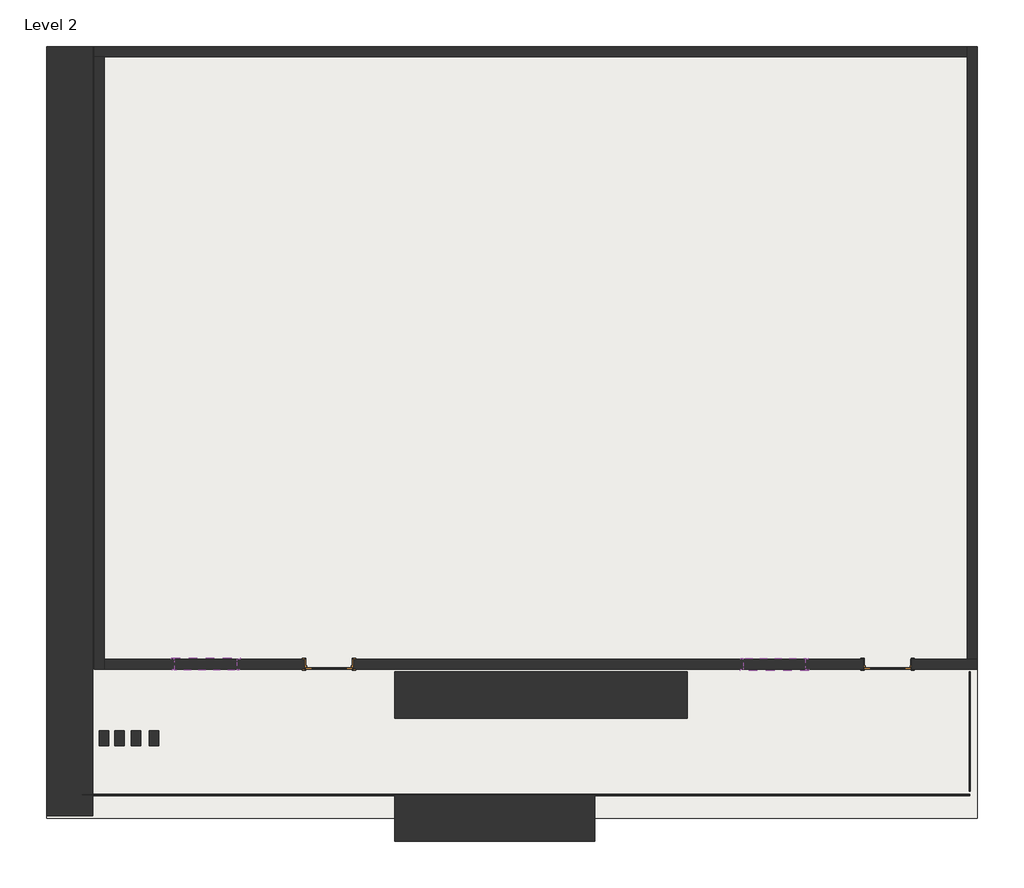
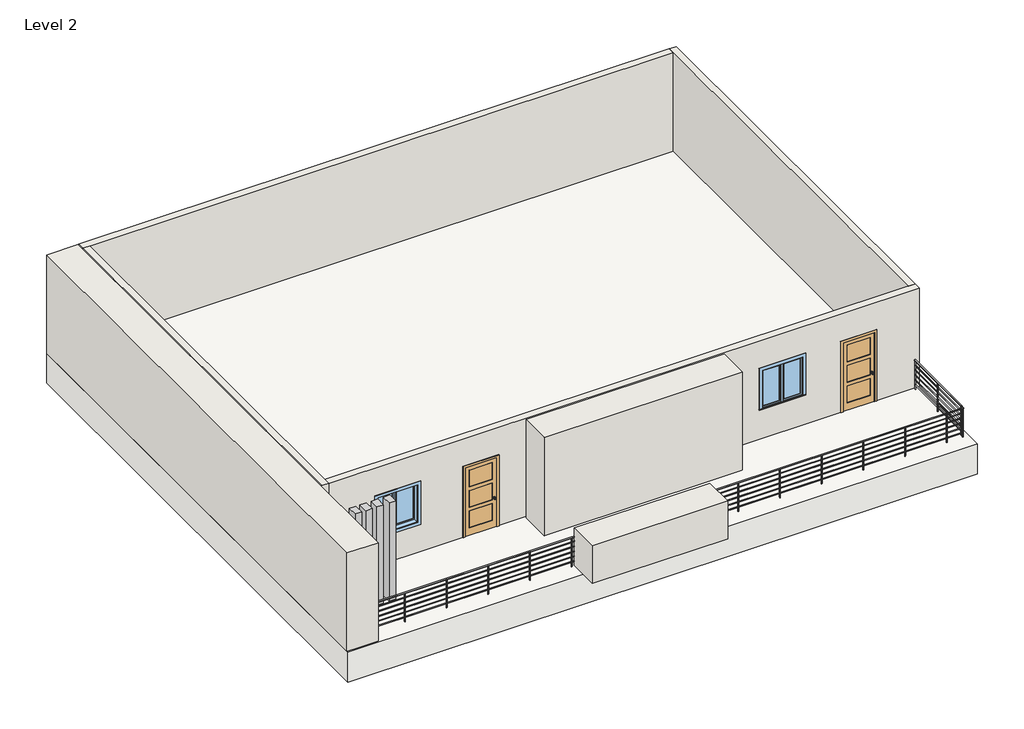
# One storey: 7 walls, 4 columns, 2 doors, 2 railings, 2 windows, 1 slab.
"""IFC4 building model written with IfcOpenShell, lengths in millimetres."""

from ifc_helpers import new_model, si_unit, point, frame, frame_2d, origin, place, context, project, spatial, polyline, circle_curve, trimmed, segment, composite_curve, outline, extrude, faceted_brep, transform, mapped, element, save
from components import wood_timber_column_8_x_12_4a74a8f5, door_54d869bf, window_3a1167bf, window_0862ab64

model = new_model("IFC4")

# Units and contexts
model_context = context("Model", 3, world=origin())
ifc_project = project(units=[si_unit("LENGTHUNIT", "METRE", prefix="MILLI")], contexts=[model_context])

# Site, building, storey
site = spatial("IfcSite", under=ifc_project)
building = spatial("IfcBuilding", under=site)
storey = spatial("IfcBuildingStorey", under=building, Name="Level 2", Elevation=3048.0)

# Columns
placement = place(None, origin())
wood_timber_column_8_x_12_shape = wood_timber_column_8_x_12_4a74a8f5(model_context)
element("IfcColumn", 1, ObjectType="Wood Timber Column : 8 x 12", at=placement, inside=storey, context=model_context, shape_type="MappedRepresentation", body=[
    mapped(wood_timber_column_8_x_12_shape, transform((-18270.7121948, 4590.8323495, 0.0), x_axis=(1.0, 0.0, 0.0), y_axis=(0.0, 1.0, 0.0), z_axis=(0.0, 0.0, 1.0))),
])
element("IfcColumn", 2, ObjectType="Wood Timber Column : 8 x 12", at=placement, inside=storey, context=model_context, shape_type="MappedRepresentation", body=[
    mapped(wood_timber_column_8_x_12_shape, transform((-18600.9121948, 4590.8323495, 0.0), x_axis=(1.0, 0.0, 0.0), y_axis=(0.0, 1.0, 0.0), z_axis=(0.0, 0.0, 1.0))),
])
element("IfcColumn", 3, ObjectType="Wood Timber Column : 8 x 12", at=placement, inside=storey, context=model_context, shape_type="MappedRepresentation", body=[
    mapped(wood_timber_column_8_x_12_shape, transform((-18905.7121948, 4590.8323495, 0.0), x_axis=(1.0, 0.0, 0.0), y_axis=(0.0, 1.0, 0.0), z_axis=(0.0, 0.0, 1.0))),
])
element("IfcColumn", 4, ObjectType="Wood Timber Column : 8 x 12", at=placement, inside=storey, context=model_context, shape_type="MappedRepresentation", body=[
    mapped(wood_timber_column_8_x_12_shape, transform((-17915.1121948, 4590.8323495, 0.0), x_axis=(1.0, 0.0, 0.0), y_axis=(0.0, 1.0, 0.0), z_axis=(0.0, 0.0, 1.0))),
])

# Doors
door_shape = door_54d869bf(model_context)
element("IfcDoor", 5, ObjectType="Door-Interior-Single-3_Panel_Vert-Wood : 36\" x 84\" 2", at=placement, inside=storey, context=model_context, shape_type="MappedRepresentation", body=[
    mapped(door_shape, transform((-3405.3621948, 6054.574368, 3946.3794859), x_axis=(-1.0, 0.0, 0.0), y_axis=(0.0, -1.0, 0.0), z_axis=(0.0, 0.0, 1.0))),
])
element("IfcDoor", 6, ObjectType="Door-Interior-Single-3_Panel_Vert-Wood : 36\" x 84\" 2", at=placement, inside=storey, context=model_context, shape_type="MappedRepresentation", body=[
    mapped(door_shape, transform((-14454.3621948, 6054.574368, 3946.3794859), x_axis=(-1.0, 0.0, 0.0), y_axis=(0.0, -1.0, 0.0), z_axis=(0.0, 0.0, 1.0))),
])

# Railings
element("IfcRailing", 7, ObjectType="Handrail - Pipe", at=placement, inside=storey, context=model_context, shape_type="SweptSolid", body=[
    extrude(outline(composite_curve([segment(trimmed(circle_curve(frame_2d((3466.949368, 4841.7294859)), 19.05), [point((3447.899368, 4841.7294859))], [point((3485.999368, 4841.7294859))], False, "CARTESIAN"), True, "CONTINUOUS"), segment(trimmed(circle_curve(frame_2d((3466.949368, 4841.7294859)), 19.05), [point((3485.999368, 4841.7294859))], [point((3447.899368, 4841.7294859))], False, "CARTESIAN"), True, "CONTINUOUS")], self_intersect=False)), frame((-19331.1621948, 0.0, 0.0), z_axis=(1.0, 0.0, 0.0), x_axis=(0.0, 1.0, 0.0)), (0.0, 0.0, 1.0), 17551.4),
    extrude(outline(composite_curve([segment(trimmed(circle_curve(frame_2d((3466.949368, 4695.6794859)), 12.7), [point((3479.649368, 4695.6794859))], [point((3454.249368, 4695.6794859))], False, "CARTESIAN"), True, "CONTINUOUS"), segment(trimmed(circle_curve(frame_2d((3466.949368, 4695.6794859)), 12.7), [point((3454.249368, 4695.6794859))], [point((3479.649368, 4695.6794859))], False, "CARTESIAN"), True, "CONTINUOUS")], self_intersect=False)), frame((-19331.1621948, 0.0, 0.0), z_axis=(1.0, 0.0, 0.0), x_axis=(0.0, 1.0, 0.0)), (0.0, 0.0, 1.0), 17551.4),
    extrude(outline(composite_curve([segment(trimmed(circle_curve(frame_2d((3466.949368, 4543.2794859)), 12.7), [point((3479.649368, 4543.2794859))], [point((3454.249368, 4543.2794859))], False, "CARTESIAN"), True, "CONTINUOUS"), segment(trimmed(circle_curve(frame_2d((3466.949368, 4543.2794859)), 12.7), [point((3454.249368, 4543.2794859))], [point((3479.649368, 4543.2794859))], False, "CARTESIAN"), True, "CONTINUOUS")], self_intersect=False)), frame((-19331.1621948, 0.0, 0.0), z_axis=(1.0, 0.0, 0.0), x_axis=(0.0, 1.0, 0.0)), (0.0, 0.0, 1.0), 17551.4),
    extrude(outline(composite_curve([segment(trimmed(circle_curve(frame_2d((3466.949368, 4390.8794859)), 12.7), [point((3479.649368, 4390.8794859))], [point((3454.249368, 4390.8794859))], False, "CARTESIAN"), True, "CONTINUOUS"), segment(trimmed(circle_curve(frame_2d((3466.949368, 4390.8794859)), 12.7), [point((3454.249368, 4390.8794859))], [point((3479.649368, 4390.8794859))], False, "CARTESIAN"), True, "CONTINUOUS")], self_intersect=False)), frame((-19331.1621948, 0.0, 0.0), z_axis=(1.0, 0.0, 0.0), x_axis=(0.0, 1.0, 0.0)), (0.0, 0.0, 1.0), 17551.4),
    extrude(outline(composite_curve([segment(trimmed(circle_curve(frame_2d((3466.949368, 4238.4794859)), 12.7), [point((3479.649368, 4238.4794859))], [point((3454.249368, 4238.4794859))], False, "CARTESIAN"), True, "CONTINUOUS"), segment(trimmed(circle_curve(frame_2d((3466.949368, 4238.4794859)), 12.7), [point((3454.249368, 4238.4794859))], [point((3479.649368, 4238.4794859))], False, "CARTESIAN"), True, "CONTINUOUS")], self_intersect=False)), frame((-19331.1621948, 0.0, 0.0), z_axis=(1.0, 0.0, 0.0), x_axis=(0.0, 1.0, 0.0)), (0.0, 0.0, 1.0), 17551.4),
    extrude(outline(composite_curve([segment(trimmed(circle_curve(frame_2d((3466.949368, 4086.0794859)), 12.7), [point((3479.649368, 4086.0794859))], [point((3454.249368, 4086.0794859))], False, "CARTESIAN"), True, "CONTINUOUS"), segment(trimmed(circle_curve(frame_2d((3466.949368, 4086.0794859)), 12.7), [point((3454.249368, 4086.0794859))], [point((3479.649368, 4086.0794859))], False, "CARTESIAN"), True, "CONTINUOUS")], self_intersect=False)), frame((-19331.1621948, 0.0, 0.0), z_axis=(1.0, 0.0, 0.0), x_axis=(0.0, 1.0, 0.0)), (0.0, 0.0, 1.0), 17551.4),
    extrude(outline(composite_curve([segment(trimmed(circle_curve(frame_2d((-2262.3621948, 3466.949368)), 12.7), [point((-2262.3621948, 3479.649368))], [point((-2262.3621948, 3454.249368))], False, "CARTESIAN"), True, "CONTINUOUS"), segment(trimmed(circle_curve(frame_2d((-2262.3621948, 3466.949368)), 12.7), [point((-2262.3621948, 3454.249368))], [point((-2262.3621948, 3479.649368))], False, "CARTESIAN"), True, "CONTINUOUS")], self_intersect=False)), frame((0.0, 0.0, 3946.3794859), z_axis=(0.0, 0.0, 1.0), x_axis=(1.0, 0.0, 0.0)), (0.0, 0.0, 1.0), 876.3),
    extrude(outline(composite_curve([segment(trimmed(circle_curve(frame_2d((-3481.5621948, 3466.949368)), 12.7), [point((-3481.5621948, 3479.649368))], [point((-3481.5621948, 3454.249368))], False, "CARTESIAN"), True, "CONTINUOUS"), segment(trimmed(circle_curve(frame_2d((-3481.5621948, 3466.949368)), 12.7), [point((-3481.5621948, 3454.249368))], [point((-3481.5621948, 3479.649368))], False, "CARTESIAN"), True, "CONTINUOUS")], self_intersect=False)), frame((0.0, 0.0, 3946.3794859), z_axis=(0.0, 0.0, 1.0), x_axis=(1.0, 0.0, 0.0)), (0.0, 0.0, 1.0), 876.3),
    extrude(outline(composite_curve([segment(trimmed(circle_curve(frame_2d((-4700.7621948, 3466.949368)), 12.7), [point((-4700.7621948, 3479.649368))], [point((-4700.7621948, 3454.249368))], False, "CARTESIAN"), True, "CONTINUOUS"), segment(trimmed(circle_curve(frame_2d((-4700.7621948, 3466.949368)), 12.7), [point((-4700.7621948, 3454.249368))], [point((-4700.7621948, 3479.649368))], False, "CARTESIAN"), True, "CONTINUOUS")], self_intersect=False)), frame((0.0, 0.0, 3946.3794859), z_axis=(0.0, 0.0, 1.0), x_axis=(1.0, 0.0, 0.0)), (0.0, 0.0, 1.0), 876.3),
    extrude(outline(composite_curve([segment(trimmed(circle_curve(frame_2d((-5919.9621948, 3466.949368)), 12.7), [point((-5919.9621948, 3479.649368))], [point((-5919.9621948, 3454.249368))], False, "CARTESIAN"), True, "CONTINUOUS"), segment(trimmed(circle_curve(frame_2d((-5919.9621948, 3466.949368)), 12.7), [point((-5919.9621948, 3454.249368))], [point((-5919.9621948, 3479.649368))], False, "CARTESIAN"), True, "CONTINUOUS")], self_intersect=False)), frame((0.0, 0.0, 3946.3794859), z_axis=(0.0, 0.0, 1.0), x_axis=(1.0, 0.0, 0.0)), (0.0, 0.0, 1.0), 876.3),
    extrude(outline(composite_curve([segment(trimmed(circle_curve(frame_2d((-7139.1621948, 3466.949368)), 12.7), [point((-7139.1621948, 3479.649368))], [point((-7139.1621948, 3454.249368))], False, "CARTESIAN"), True, "CONTINUOUS"), segment(trimmed(circle_curve(frame_2d((-7139.1621948, 3466.949368)), 12.7), [point((-7139.1621948, 3454.249368))], [point((-7139.1621948, 3479.649368))], False, "CARTESIAN"), True, "CONTINUOUS")], self_intersect=False)), frame((0.0, 0.0, 3946.3794859), z_axis=(0.0, 0.0, 1.0), x_axis=(1.0, 0.0, 0.0)), (0.0, 0.0, 1.0), 876.3),
    extrude(outline(composite_curve([segment(trimmed(circle_curve(frame_2d((-8358.3621948, 3466.949368)), 12.7), [point((-8358.3621948, 3479.649368))], [point((-8358.3621948, 3454.249368))], False, "CARTESIAN"), True, "CONTINUOUS"), segment(trimmed(circle_curve(frame_2d((-8358.3621948, 3466.949368)), 12.7), [point((-8358.3621948, 3454.249368))], [point((-8358.3621948, 3479.649368))], False, "CARTESIAN"), True, "CONTINUOUS")], self_intersect=False)), frame((0.0, 0.0, 3946.3794859), z_axis=(0.0, 0.0, 1.0), x_axis=(1.0, 0.0, 0.0)), (0.0, 0.0, 1.0), 876.3),
    extrude(outline(composite_curve([segment(trimmed(circle_curve(frame_2d((-9577.5621948, 3466.949368)), 12.7), [point((-9577.5621948, 3479.649368))], [point((-9577.5621948, 3454.249368))], False, "CARTESIAN"), True, "CONTINUOUS"), segment(trimmed(circle_curve(frame_2d((-9577.5621948, 3466.949368)), 12.7), [point((-9577.5621948, 3454.249368))], [point((-9577.5621948, 3479.649368))], False, "CARTESIAN"), True, "CONTINUOUS")], self_intersect=False)), frame((0.0, 0.0, 3946.3794859), z_axis=(0.0, 0.0, 1.0), x_axis=(1.0, 0.0, 0.0)), (0.0, 0.0, 1.0), 876.3),
    extrude(outline(composite_curve([segment(trimmed(circle_curve(frame_2d((-10796.7621948, 3466.949368)), 12.7), [point((-10796.7621948, 3479.649368))], [point((-10796.7621948, 3454.249368))], False, "CARTESIAN"), True, "CONTINUOUS"), segment(trimmed(circle_curve(frame_2d((-10796.7621948, 3466.949368)), 12.7), [point((-10796.7621948, 3454.249368))], [point((-10796.7621948, 3479.649368))], False, "CARTESIAN"), True, "CONTINUOUS")], self_intersect=False)), frame((0.0, 0.0, 3946.3794859), z_axis=(0.0, 0.0, 1.0), x_axis=(1.0, 0.0, 0.0)), (0.0, 0.0, 1.0), 876.3),
    extrude(outline(composite_curve([segment(trimmed(circle_curve(frame_2d((-12015.9621948, 3466.949368)), 12.7), [point((-12015.9621948, 3479.649368))], [point((-12015.9621948, 3454.249368))], False, "CARTESIAN"), True, "CONTINUOUS"), segment(trimmed(circle_curve(frame_2d((-12015.9621948, 3466.949368)), 12.7), [point((-12015.9621948, 3454.249368))], [point((-12015.9621948, 3479.649368))], False, "CARTESIAN"), True, "CONTINUOUS")], self_intersect=False)), frame((0.0, 0.0, 3946.3794859), z_axis=(0.0, 0.0, 1.0), x_axis=(1.0, 0.0, 0.0)), (0.0, 0.0, 1.0), 876.3),
    extrude(outline(composite_curve([segment(trimmed(circle_curve(frame_2d((-13235.1621948, 3466.949368)), 12.7), [point((-13235.1621948, 3479.649368))], [point((-13235.1621948, 3454.249368))], False, "CARTESIAN"), True, "CONTINUOUS"), segment(trimmed(circle_curve(frame_2d((-13235.1621948, 3466.949368)), 12.7), [point((-13235.1621948, 3454.249368))], [point((-13235.1621948, 3479.649368))], False, "CARTESIAN"), True, "CONTINUOUS")], self_intersect=False)), frame((0.0, 0.0, 3946.3794859), z_axis=(0.0, 0.0, 1.0), x_axis=(1.0, 0.0, 0.0)), (0.0, 0.0, 1.0), 876.3),
    extrude(outline(composite_curve([segment(trimmed(circle_curve(frame_2d((-14454.3621948, 3466.949368)), 12.7), [point((-14454.3621948, 3479.649368))], [point((-14454.3621948, 3454.249368))], False, "CARTESIAN"), True, "CONTINUOUS"), segment(trimmed(circle_curve(frame_2d((-14454.3621948, 3466.949368)), 12.7), [point((-14454.3621948, 3454.249368))], [point((-14454.3621948, 3479.649368))], False, "CARTESIAN"), True, "CONTINUOUS")], self_intersect=False)), frame((0.0, 0.0, 3946.3794859), z_axis=(0.0, 0.0, 1.0), x_axis=(1.0, 0.0, 0.0)), (0.0, 0.0, 1.0), 876.3),
    extrude(outline(composite_curve([segment(trimmed(circle_curve(frame_2d((-15673.5621948, 3466.949368)), 12.7), [point((-15673.5621948, 3479.649368))], [point((-15673.5621948, 3454.249368))], False, "CARTESIAN"), True, "CONTINUOUS"), segment(trimmed(circle_curve(frame_2d((-15673.5621948, 3466.949368)), 12.7), [point((-15673.5621948, 3454.249368))], [point((-15673.5621948, 3479.649368))], False, "CARTESIAN"), True, "CONTINUOUS")], self_intersect=False)), frame((0.0, 0.0, 3946.3794859), z_axis=(0.0, 0.0, 1.0), x_axis=(1.0, 0.0, 0.0)), (0.0, 0.0, 1.0), 876.3),
    extrude(outline(composite_curve([segment(trimmed(circle_curve(frame_2d((-16892.7621948, 3466.949368)), 12.7), [point((-16892.7621948, 3479.649368))], [point((-16892.7621948, 3454.249368))], False, "CARTESIAN"), True, "CONTINUOUS"), segment(trimmed(circle_curve(frame_2d((-16892.7621948, 3466.949368)), 12.7), [point((-16892.7621948, 3454.249368))], [point((-16892.7621948, 3479.649368))], False, "CARTESIAN"), True, "CONTINUOUS")], self_intersect=False)), frame((0.0, 0.0, 3946.3794859), z_axis=(0.0, 0.0, 1.0), x_axis=(1.0, 0.0, 0.0)), (0.0, 0.0, 1.0), 876.3),
    extrude(outline(composite_curve([segment(trimmed(circle_curve(frame_2d((-18111.9621948, 3466.949368)), 12.7), [point((-18111.9621948, 3479.649368))], [point((-18111.9621948, 3454.249368))], False, "CARTESIAN"), True, "CONTINUOUS"), segment(trimmed(circle_curve(frame_2d((-18111.9621948, 3466.949368)), 12.7), [point((-18111.9621948, 3454.249368))], [point((-18111.9621948, 3479.649368))], False, "CARTESIAN"), True, "CONTINUOUS")], self_intersect=False)), frame((0.0, 0.0, 3946.3794859), z_axis=(0.0, 0.0, 1.0), x_axis=(1.0, 0.0, 0.0)), (0.0, 0.0, 1.0), 876.3),
    extrude(outline(composite_curve([segment(trimmed(circle_curve(frame_2d((-1792.4621948, 3466.949368)), 12.7), [point((-1792.4621948, 3479.649368))], [point((-1792.4621948, 3454.249368))], False, "CARTESIAN"), True, "CONTINUOUS"), segment(trimmed(circle_curve(frame_2d((-1792.4621948, 3466.949368)), 12.7), [point((-1792.4621948, 3454.249368))], [point((-1792.4621948, 3479.649368))], False, "CARTESIAN"), True, "CONTINUOUS")], self_intersect=False)), frame((0.0, 0.0, 3946.3794859), z_axis=(0.0, 0.0, 1.0), x_axis=(1.0, 0.0, 0.0)), (0.0, 0.0, 1.0), 876.3),
    extrude(outline(composite_curve([segment(trimmed(circle_curve(frame_2d((-19318.4621948, 3466.949368)), 12.7), [point((-19318.4621948, 3479.649368))], [point((-19318.4621948, 3454.249368))], False, "CARTESIAN"), True, "CONTINUOUS"), segment(trimmed(circle_curve(frame_2d((-19318.4621948, 3466.949368)), 12.7), [point((-19318.4621948, 3454.249368))], [point((-19318.4621948, 3479.649368))], False, "CARTESIAN"), True, "CONTINUOUS")], self_intersect=False)), frame((0.0, 0.0, 3946.3794859), z_axis=(0.0, 0.0, 1.0), x_axis=(1.0, 0.0, 0.0)), (0.0, 0.0, 1.0), 876.3),
])
element("IfcRailing", 8, ObjectType="Handrail - Pipe", at=placement, inside=storey, context=model_context, shape_type="SweptSolid", body=[
    extrude(outline(composite_curve([segment(trimmed(circle_curve(frame_2d((4841.7294859, -1779.7621948)), 19.05), [point((4841.7294859, -1760.7121948))], [point((4841.7294859, -1798.8121948))], False, "CARTESIAN"), True, "CONTINUOUS"), segment(trimmed(circle_curve(frame_2d((4841.7294859, -1779.7621948)), 19.05), [point((4841.7294859, -1798.8121948))], [point((4841.7294859, -1760.7121948))], False, "CARTESIAN"), True, "CONTINUOUS")], self_intersect=False)), frame((0.0, 3543.149368, 0.0), z_axis=(0.0, 1.0, 0.0), x_axis=(0.0, 0.0, 1.0)), (0.0, 0.0, 1.0), 2362.2),
    extrude(outline(composite_curve([segment(trimmed(circle_curve(frame_2d((4695.6794859, -1779.7621948)), 12.7), [point((4695.6794859, -1792.4621948))], [point((4695.6794859, -1767.0621948))], False, "CARTESIAN"), True, "CONTINUOUS"), segment(trimmed(circle_curve(frame_2d((4695.6794859, -1779.7621948)), 12.7), [point((4695.6794859, -1767.0621948))], [point((4695.6794859, -1792.4621948))], False, "CARTESIAN"), True, "CONTINUOUS")], self_intersect=False)), frame((0.0, 3543.149368, 0.0), z_axis=(0.0, 1.0, 0.0), x_axis=(0.0, 0.0, 1.0)), (0.0, 0.0, 1.0), 2362.2),
    extrude(outline(composite_curve([segment(trimmed(circle_curve(frame_2d((4543.2794859, -1779.7621948)), 12.7), [point((4543.2794859, -1792.4621948))], [point((4543.2794859, -1767.0621948))], False, "CARTESIAN"), True, "CONTINUOUS"), segment(trimmed(circle_curve(frame_2d((4543.2794859, -1779.7621948)), 12.7), [point((4543.2794859, -1767.0621948))], [point((4543.2794859, -1792.4621948))], False, "CARTESIAN"), True, "CONTINUOUS")], self_intersect=False)), frame((0.0, 3543.149368, 0.0), z_axis=(0.0, 1.0, 0.0), x_axis=(0.0, 0.0, 1.0)), (0.0, 0.0, 1.0), 2362.2),
    extrude(outline(composite_curve([segment(trimmed(circle_curve(frame_2d((4390.8794859, -1779.7621948)), 12.7), [point((4390.8794859, -1792.4621948))], [point((4390.8794859, -1767.0621948))], False, "CARTESIAN"), True, "CONTINUOUS"), segment(trimmed(circle_curve(frame_2d((4390.8794859, -1779.7621948)), 12.7), [point((4390.8794859, -1767.0621948))], [point((4390.8794859, -1792.4621948))], False, "CARTESIAN"), True, "CONTINUOUS")], self_intersect=False)), frame((0.0, 3543.149368, 0.0), z_axis=(0.0, 1.0, 0.0), x_axis=(0.0, 0.0, 1.0)), (0.0, 0.0, 1.0), 2362.2),
    extrude(outline(composite_curve([segment(trimmed(circle_curve(frame_2d((4238.4794859, -1779.7621948)), 12.7), [point((4238.4794859, -1792.4621948))], [point((4238.4794859, -1767.0621948))], False, "CARTESIAN"), True, "CONTINUOUS"), segment(trimmed(circle_curve(frame_2d((4238.4794859, -1779.7621948)), 12.7), [point((4238.4794859, -1767.0621948))], [point((4238.4794859, -1792.4621948))], False, "CARTESIAN"), True, "CONTINUOUS")], self_intersect=False)), frame((0.0, 3543.149368, 0.0), z_axis=(0.0, 1.0, 0.0), x_axis=(0.0, 0.0, 1.0)), (0.0, 0.0, 1.0), 2362.2),
    extrude(outline(composite_curve([segment(trimmed(circle_curve(frame_2d((4086.0794859, -1779.7621948)), 12.7), [point((4086.0794859, -1792.4621948))], [point((4086.0794859, -1767.0621948))], False, "CARTESIAN"), True, "CONTINUOUS"), segment(trimmed(circle_curve(frame_2d((4086.0794859, -1779.7621948)), 12.7), [point((4086.0794859, -1767.0621948))], [point((4086.0794859, -1792.4621948))], False, "CARTESIAN"), True, "CONTINUOUS")], self_intersect=False)), frame((0.0, 3543.149368, 0.0), z_axis=(0.0, 1.0, 0.0), x_axis=(0.0, 0.0, 1.0)), (0.0, 0.0, 1.0), 2362.2),
    extrude(outline(composite_curve([segment(trimmed(circle_curve(frame_2d((-1779.7621948, 4762.349368)), 12.7), [point((-1792.4621948, 4762.349368))], [point((-1767.0621948, 4762.349368))], False, "CARTESIAN"), True, "CONTINUOUS"), segment(trimmed(circle_curve(frame_2d((-1779.7621948, 4762.349368)), 12.7), [point((-1767.0621948, 4762.349368))], [point((-1792.4621948, 4762.349368))], False, "CARTESIAN"), True, "CONTINUOUS")], self_intersect=False)), frame((0.0, 0.0, 3946.3794859), z_axis=(0.0, 0.0, 1.0), x_axis=(1.0, 0.0, 0.0)), (0.0, 0.0, 1.0), 876.3),
    extrude(outline(composite_curve([segment(trimmed(circle_curve(frame_2d((-1779.7621948, 5892.649368)), 12.7), [point((-1792.4621948, 5892.649368))], [point((-1767.0621948, 5892.649368))], False, "CARTESIAN"), True, "CONTINUOUS"), segment(trimmed(circle_curve(frame_2d((-1779.7621948, 5892.649368)), 12.7), [point((-1767.0621948, 5892.649368))], [point((-1792.4621948, 5892.649368))], False, "CARTESIAN"), True, "CONTINUOUS")], self_intersect=False)), frame((0.0, 0.0, 3946.3794859), z_axis=(0.0, 0.0, 1.0), x_axis=(1.0, 0.0, 0.0)), (0.0, 0.0, 1.0), 876.3),
    extrude(outline(composite_curve([segment(trimmed(circle_curve(frame_2d((-1779.7621948, 3555.849368)), 12.7), [point((-1792.4621948, 3555.849368))], [point((-1767.0621948, 3555.849368))], False, "CARTESIAN"), True, "CONTINUOUS"), segment(trimmed(circle_curve(frame_2d((-1779.7621948, 3555.849368)), 12.7), [point((-1767.0621948, 3555.849368))], [point((-1792.4621948, 3555.849368))], False, "CARTESIAN"), True, "CONTINUOUS")], self_intersect=False)), frame((0.0, 0.0, 3946.3794859), z_axis=(0.0, 0.0, 1.0), x_axis=(1.0, 0.0, 0.0)), (0.0, 0.0, 1.0), 876.3),
])

# Slab
element("IfcSlab", 9, ObjectType="Generic - 3'", at=placement, inside=storey, context=model_context, shape_type="SweptSolid", body=[
    extrude(outline(polyline([(-1627.3621948, 18275.149368), (-1627.3621948, 3009.749368), (-20042.3621948, 3009.749368), (-20042.3621948, 18275.149368), (-1627.3621948, 18275.149368)])), frame((0.0, 0.0, 3031.9794859), z_axis=(0.0, 0.0, 1.0), x_axis=(1.0, 0.0, 0.0)), (0.0, 0.0, 1.0), 914.4),
])

# Walls
element("IfcWall", 10, ObjectType="Generic - 3' 2", at=placement, inside=storey, context=model_context, shape_type="SweptSolid", body=[
    extrude(outline(polyline([(-7367.7621948, 4990.949368), (-13158.9621948, 4990.949368), (-13158.9621948, 5905.349368), (-7367.7621948, 5905.349368), (-7367.7621948, 4990.949368)])), frame((0.0, 0.0, 3946.3794859), z_axis=(0.0, 0.0, 1.0), x_axis=(1.0, 0.0, 0.0)), (0.0, 0.0, 1.0), 3048.0),
])
element("IfcWall", 11, ObjectType="Generic - 3' 4", at=placement, inside=storey, context=model_context, shape_type="SweptSolid", body=[
    extrude(outline(polyline([(-9196.5621948, 2552.549368), (-13158.9621948, 2552.549368), (-13158.9621948, 3466.949368), (-9196.5621948, 3466.949368), (-9196.5621948, 2552.549368)])), frame((0.0, 0.0, 3946.3794859), z_axis=(0.0, 0.0, 1.0), x_axis=(1.0, 0.0, 0.0)), (0.0, 0.0, 1.0), 1165.3811612),
])
element("IfcWall", 12, ObjectType="Generic - 3' 4", at=placement, inside=storey, context=model_context, shape_type="SweptSolid", body=[
    extrude(outline(polyline([(-20042.3621948, 3060.549368), (-20042.3621948, 18275.149368), (-19127.9621948, 18275.149368), (-19127.9621948, 3060.549368), (-20042.3621948, 3060.549368)])), frame((0.0, 0.0, 3946.3794859), z_axis=(0.0, 0.0, 1.0), x_axis=(1.0, 0.0, 0.0)), (0.0, 0.0, 1.0), 3048.0),
])
element("IfcWall", 13, ObjectType="Generic - 8\"", at=placement, inside=storey, context=model_context, shape_type="Brep", body=[
    faceted_brep([(-19102.5621948, 18071.949368, 3946.3794859), (-18899.3621948, 18071.949368, 3946.3794859), (-1830.5621948, 18071.949368, 3946.3794859), (-1830.5621948, 18071.949368, 6994.3794859), (-18899.3621948, 18071.949368, 6994.3794859), (-19102.5621948, 18071.949368, 6994.3794859), (-19102.5621948, 18275.149368, 3946.3794859), (-19102.5621948, 18275.149368, 6994.3794859), (-1830.5621948, 18275.149368, 6994.3794859), (-1830.5621948, 18275.149368, 3946.3794859)], [[[0, 1, 2, 3, 4, 5]], [[6, 7, 8, 9]], [[2, 1, 0, 6, 9]], [[5, 4, 3, 8, 7]], [[0, 5, 7, 6]], [[3, 2, 9, 8]]]),
])
element("IfcWall", 14, ObjectType="Generic - 8\"", at=placement, inside=storey, context=model_context, shape_type="Brep", body=[
    faceted_brep([(-18899.3621948, 6159.349368, 6994.3794859), (-1830.5621948, 6159.349368, 6994.3794859), (-1627.3621948, 6159.349368, 6994.3794859), (-1627.3621948, 6159.349368, 3946.3794859), (-1830.5621948, 6159.349368, 3946.3794859), (-2922.7621948, 6159.349368, 3946.3794859), (-2922.7621948, 6159.349368, 6105.3794859), (-3887.9621948, 6159.349368, 6105.3794859), (-3887.9621948, 6159.349368, 3946.3794859), (-13971.7621948, 6159.349368, 3946.3794859), (-13971.7621948, 6159.349368, 6105.3794859), (-14936.9621948, 6159.349368, 6105.3794859), (-14936.9621948, 6159.349368, 3946.3794859), (-18899.3621948, 6159.349368, 3946.3794859), (-17502.3621948, 6159.349368, 6079.9794859), (-17502.3621948, 6159.349368, 4860.7794859), (-16283.1621948, 6159.349368, 4860.7794859), (-16283.1621948, 6159.349368, 6079.9794859), (-6250.1621948, 6159.349368, 6079.9794859), (-6250.1621948, 6159.349368, 4860.7794859), (-5030.9621948, 6159.349368, 4860.7794859), (-5030.9621948, 6159.349368, 6079.9794859), (-1627.3621948, 5956.149368, 6994.3794859), (-18899.3621948, 5956.149368, 6994.3794859), (-18899.3621948, 5956.149368, 3946.3794859), (-14936.9621948, 5956.149368, 3946.3794859), (-14936.9621948, 5956.149368, 6105.3794859), (-13971.7621948, 5956.149368, 6105.3794859), (-13971.7621948, 5956.149368, 3946.3794859), (-3887.9621948, 5956.149368, 3946.3794859), (-3887.9621948, 5956.149368, 6105.3794859), (-2922.7621948, 5956.149368, 6105.3794859), (-2922.7621948, 5956.149368, 3946.3794859), (-1627.3621948, 5956.149368, 3946.3794859), (-17502.3621948, 5956.149368, 6079.9794859), (-16283.1621948, 5956.149368, 6079.9794859), (-16283.1621948, 5956.149368, 4860.7794859), (-17502.3621948, 5956.149368, 4860.7794859), (-6250.1621948, 5956.149368, 6079.9794859), (-5030.9621948, 5956.149368, 6079.9794859), (-5030.9621948, 5956.149368, 4860.7794859), (-6250.1621948, 5956.149368, 4860.7794859)], [[[0, 1, 2, 3, 4, 5, 6, 7, 8, 9, 10, 11, 12, 13], [14, 15, 16, 17], [18, 19, 20, 21]], [[22, 23, 24, 25, 26, 27, 28, 29, 30, 31, 32, 33], [34, 35, 36, 37], [38, 39, 40, 41]], [[3, 33, 32, 5, 4]], [[8, 29, 28, 9]], [[24, 13, 12, 25]], [[2, 1, 0, 23, 22]], [[3, 2, 22, 33]], [[7, 30, 29, 8]], [[30, 7, 6, 31]], [[31, 6, 5, 32]], [[11, 26, 25, 12]], [[26, 11, 10, 27]], [[27, 10, 9, 28]], [[15, 14, 34, 37]], [[16, 15, 37, 36]], [[17, 16, 36, 35]], [[14, 17, 35, 34]], [[19, 18, 38, 41]], [[20, 19, 41, 40]], [[21, 20, 40, 39]], [[18, 21, 39, 38]], [[0, 13, 24, 23]]]),
])
element("IfcWall", 15, ObjectType="Generic - 8\"", at=placement, inside=storey, context=model_context, shape_type="Brep", body=[
    faceted_brep([(-1830.5621948, 18275.149368, 3946.3794859), (-1830.5621948, 18071.949368, 3946.3794859), (-1830.5621948, 6159.349368, 3946.3794859), (-1830.5621948, 6159.349368, 6994.3794859), (-1830.5621948, 18071.949368, 6994.3794859), (-1830.5621948, 18275.149368, 6994.3794859), (-1627.3621948, 18275.149368, 3946.3794859), (-1627.3621948, 18275.149368, 6994.3794859), (-1627.3621948, 6159.349368, 6994.3794859), (-1627.3621948, 6159.349368, 3946.3794859)], [[[0, 1, 2, 3, 4, 5]], [[6, 7, 8, 9]], [[2, 1, 0, 6, 9]], [[5, 4, 3, 8, 7]], [[0, 5, 7, 6]], [[3, 2, 9, 8]]]),
])
element("IfcWall", 16, ObjectType="Generic - 8\"", at=placement, inside=storey, context=model_context, shape_type="Brep", body=[
    faceted_brep([(-18899.3621948, 5956.149368, 3946.3794859), (-18899.3621948, 6159.349368, 3946.3794859), (-18899.3621948, 18071.949368, 3946.3794859), (-18899.3621948, 18071.949368, 6994.3794859), (-18899.3621948, 6159.349368, 6994.3794859), (-18899.3621948, 5956.149368, 6994.3794859), (-19102.5621948, 5956.149368, 3946.3794859), (-19102.5621948, 5956.149368, 6994.3794859), (-19102.5621948, 18071.949368, 6994.3794859), (-19102.5621948, 18071.949368, 3946.3794859)], [[[0, 1, 2, 3, 4, 5]], [[6, 7, 8, 9]], [[2, 1, 0, 6, 9]], [[5, 4, 3, 8, 7]], [[3, 2, 9, 8]], [[0, 5, 7, 6]]]),
])

# Windows
window_shape = window_3a1167bf(model_context)
element("IfcWindow", 17, ObjectType="Casement Dbl with Trim : 48\" x 48\"", at=placement, inside=storey, context=model_context, shape_type="MappedRepresentation", body=[
    mapped(window_shape, transform((-16892.7621948, 6038.699368, 3946.3794859), x_axis=(-1.0, 0.0, 0.0), y_axis=(0.0, -1.0, 0.0), z_axis=(0.0, 0.0, 1.0))),
])
window_2_shape = window_0862ab64(model_context)
element("IfcWindow", 18, ObjectType="Casement Dbl with Trim : 48\" x 48\" 2", at=placement, inside=storey, context=model_context, shape_type="MappedRepresentation", body=[
    mapped(window_2_shape, transform((-5640.5621948, 6076.799368, 3946.3794859), x_axis=(-1.0, 0.0, 0.0), y_axis=(0.0, -1.0, 0.0), z_axis=(0.0, 0.0, 1.0))),
])

save(model, "model.ifc")

# Revit data of these elements
# Type "Wood Timber Column : 8 x 12"
#   Assembly Code = "B1010200"
#   Depth = 0' - 11 1/2"
#   Width = 0' - 7 1/2"
#   Material = Softwood, Lumber
# Type "Door-Interior-Single-3_Panel_Vert-Wood : 36\" x 84\" 2"
#   Type Mark = "11"
#   Assembly Code = "C1020300"
#   Analytic Construction = "Wooden"
#   Top Rail = 0' - 4 11/16"
#   Thickness = 0' - 1 3/8"
#   Thermal Resistance (R) = 2.5876 (h·ft²·°F)/BTU
#   Swing Angle [instance default] = 90.00°
#   Stiles = 0' - 4 3/4"
#   Rough Width = 3' - 2"
#   Rough Height = 7' - 1"
#   Intermediate Rail = 0' - 4 1/2"
#   Height = 7' - 0"
#   Width = 3' - 0"
#   Heat Transfer Coefficient (U) = 0.3865 BTU/(h·ft²·°F)
#   Bottom Rail = 0' - 9 1/8"
#   Trim Material = Cherry
#   Panel Material = Door - Panel
#   Frame Material = Door - Panel
#   Door Handle Material = Aluminum
#   Visual Light Transmittance = 0
#   Solar Heat Gain Coefficient = 0
#   Wall Closure = (empty or 0)
#   Function = (empty or 0)
# Type "Handrail - Pipe"
#   Assembly Code = "C2010400"
#   built-in parameter 1008612 = 0.0416667 (stored number, unit not read)
#   built-in parameter 1008611 = 0.0833333 (stored number, unit not read)
#   built-in parameter 1008609 = 4 (stored number, unit not read)
#   built-in parameter 1008604 = 0.166667 (stored number, unit not read)
#   built-in parameter 1008603 = 0.166667 (stored number, unit not read)
#   Railing Height = 3' - 0"
#   built-in parameter 1008630 = 2
#   built-in parameter 1008610 = 1
#   built-in parameter 1008605 = 1
#   built-in parameter 1008618 = Baluster - Round : 1"
# Type "Generic - 3'"
#   Assembly Code = "B1010"
#   Function = 0
#   Layers, outside or top first: 3' - 0" "Parking Stripe" (function 1)
# Type "Generic - 3' 2"
#   Assembly Code = "B2010"
#   Layers, outside or top first: 3' - 0" "Asphalt Shingle" (function 1)
# Type "Generic - 3' 4"
#   Assembly Code = "B2010"
#   Layers, outside or top first: 3' - 0" "Parking Stripe" (function 1)
# Type "Generic - 8\""
#   Assembly Code = "B2010"
#   Layers, outside or top first: 0' - 8" "Paint - Sienna" (function 1)
# Type "Casement Dbl with Trim : 48\" x 48\""
#   Type Mark = "10"
#   Construction Type Id = "GSP4R"
#   Assembly Code = "B2020100"
#   Analytic Construction = "1/8 in Pilkington single glazing"
#   Visual Light Transmittance = 0.9
#   Thermal Resistance (R) = 1.53941 (h·ft²·°F)/BTU
#   Solar Heat Gain Coefficient = 0.78
#   Heat Transfer Coefficient (U) = 0.6496 BTU/(h·ft²·°F)
#   Height = 4' - 0"
#   Default Sill Height = 3' - 0"
#   Trim Projection - Ext. = 0' - 0 1/2"
#   Trim Projection - Int. = 0' - 0 3/4"
#   Trim Width - Exterior = 0' - 3 1/2"
#   Trim Width - Interior = 0' - 3 1/2"
#   Width = 4' - 0"
#   Window Inset = 0' - 0 3/4"
#   Define Thermal Properties by = 1
#   Glass Pane Material = Glass
#   Sash Material = Sash
#   Trim Exterior Material = Trim
#   Trim Interior Material = Trim
#   Wall Closure = (empty or 0)
# Type "Casement Dbl with Trim : 48\" x 48\" 2"
#   Type Mark = "13"
#   Construction Type Id = "GSP4R"
#   Assembly Code = "B2020100"
#   Analytic Construction = "1/8 in Pilkington single glazing"
#   Visual Light Transmittance = 0.9
#   Thermal Resistance (R) = 1.53941 (h·ft²·°F)/BTU
#   Solar Heat Gain Coefficient = 0.78
#   Heat Transfer Coefficient (U) = 0.6496 BTU/(h·ft²·°F)
#   Height = 4' - 0"
#   Default Sill Height = 3' - 0"
#   Trim Projection - Ext. = 0' - 0 1/2"
#   Trim Projection - Int. = 0' - 0 3/4"
#   Trim Width - Exterior = 0' - 3 1/2"
#   Trim Width - Interior = 0' - 3 1/2"
#   Width = 4' - 0"
#   Window Inset = 0' - 0 3/4"
#   Define Thermal Properties by = 1
#   Glass Pane Material = Glass, Clear Glazing
#   Sash Material = Copper
#   Trim Exterior Material = Earth
#   Trim Interior Material = Earth
#   Wall Closure = (empty or 0)
# Elements 1, 2, 3, 4 (IfcColumn, "Wood Timber Column : 8 x 12")
#   Phase Created = New Construction
#   Materials on its faces: "Softwood, Lumber"
# Elements 5, 6 (IfcDoor, "Door-Interior-Single-3_Panel_Vert-Wood : 36\" x 84\" 2")
#   Swing Angle = 90.00°
#   Phase Created = New Construction
#   Materials on its faces: "Door - Panel", "Aluminum", "Cherry"
# Elements 7, 8 (IfcRailing, "Handrail - Pipe")
#   built-in parameter 1008621 = 2.94744 (stored number, unit not read)
#   Phase Created = New Construction
# Element 9 (IfcSlab, "Generic - 3'")
#   Height Offset From Level = 2' - 11.36927"
#   Phase Created = New Construction
#   Materials on its faces: "Parking Stripe"
# Element 10 (IfcWall, "Generic - 3' 2")
#   built-in parameter 1001111 = 2' - 11.36927"
#   Top Offset = 0' - 0"
#   Base Offset = 2' - 11.36927"
#   Unconnected Height = 10' - 0"
#   wall height = 10' - 0"
#   Phase Created = New Construction
#   Base Constraint = Level 2
#   Materials on its faces: "Asphalt Shingle"
# Element 11 (IfcWall, "Generic - 3' 4")
#   built-in parameter 1001111 = 2' - 11.36927"
#   Top Offset = 0' - 0"
#   Base Offset = 2' - 11.36927"
#   Unconnected Height = 3' - 9.88115"
#   wall height = 3' - 9.88115"
#   Phase Created = New Construction
#   Base Constraint = Level 2
#   Materials on its faces: "Parking Stripe"
# Element 12 (IfcWall, "Generic - 3' 4")
#   built-in parameter 1001111 = 2' - 11.36927"
#   Top Offset = 0' - 0"
#   Base Offset = 2' - 11.36927"
#   Unconnected Height = 10' - 0"
#   wall height = 10' - 0"
#   Phase Created = New Construction
#   Base Constraint = Level 2
#   Materials on its faces: "Parking Stripe"
# Elements 13, 14, 15, 16 (IfcWall, "Generic - 8\"")
#   built-in parameter 1001111 = 2' - 11.36927"
#   Top Offset = 0' - 0"
#   Base Offset = 2' - 11.36927"
#   Unconnected Height = 10' - 0"
#   wall height = 10' - 0"
#   Phase Created = New Construction
#   Base Constraint = Level 2
#   Materials on its faces: "Paint - Sienna"
# Element 17 (IfcWindow, "Casement Dbl with Trim : 48\" x 48\"")
#   Mark = "6"
#   Phase Created = New Construction
#   Materials on its faces: "Sash", "Trim", "Glass"
# Element 18 (IfcWindow, "Casement Dbl with Trim : 48\" x 48\" 2")
#   Mark = "7"
#   Phase Created = New Construction
#   Materials on its faces: "Copper", "Earth", "Glass, Clear Glazing"
# Materials
#   "Softwood, Lumber": class "Wood", colour RGB 223 192 134, transparency 0, Description = "Pinus Echinata", Cost = 0
#   "Cherry": class "Wood", colour RGB 226 177 128, transparency 0, Description = "Prunus Serotina", Cost = 0
#   "Door - Panel": class "Wood", colour RGB 210 159 95, transparency 0
#   "Aluminum": class "Metal", colour RGB 247 247 247, transparency 0, Description = "Aluminum 6061", Cost = 0
#   "Parking Stripe": class "Paint", colour RGB 255 221 187, transparency 0, Cost = 0
#   "Asphalt Shingle": class "Generic", colour RGB 155 155 155, transparency 0, Description = "Asphalt roofing shingle", Cost = 0
#   "Paint - Sienna": colour RGB 255 255 255, transparency 0, Cost = 0
#   "Glass": class "Glass", colour RGB 0 128 192, transparency 0.75, Description = "Soda Lime Glass", Cost = 0
#   "Sash": class "Wood", colour RGB 224 178 126, transparency 0
#   "Trim": class "Wood", colour RGB 224 178 126, transparency 0
#   "Glass, Clear Glazing": class "Glass", colour RGB 0 128 192, transparency 0.75, Description = "Clear glazing", Cost = 0
#   "Copper": class "Metal", colour RGB 0 0 0, transparency 0, Description = "Copper, matte finish", Cost = 0
#   "Earth": class "Generic", colour RGB 97 75 62, transparency 0, Description = "Soil", Cost = 0
